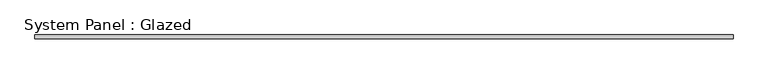
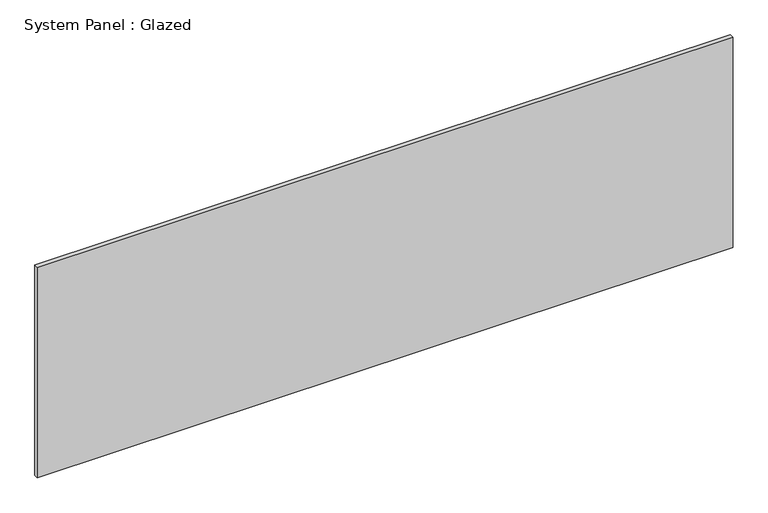
"""IFC4 building model written with IfcOpenShell, lengths in millimetres: plate geometry, System Panel : Glazed."""

from ifc_helpers import new_model, si_unit, origin, origin_with_axes, place, context, project, spatial, polyline, outline, extrude, source, transform, mapped, element, save


def system_panel_glazed_c13b8b16(model_context):
    return source(origin(), model_context, "Body", "SweptSolid", [
        extrude(outline(polyline([(2283.593154, 19.05), (-2283.593154, 19.05), (-2283.593154, 44.45), (2283.593154, 44.45), (2283.593154, 19.05)])), origin_with_axes(), (0.0, 0.0, 1.0), 1460.5),
    ])


if __name__ == "__main__":
    model = new_model("IFC4")
    model_context = context("Model", 3, world=origin())
    ifc_project = project(units=[si_unit("LENGTHUNIT", "METRE", prefix="MILLI")], contexts=[model_context])
    site = spatial("IfcSite", under=ifc_project)
    building = spatial("IfcBuilding", under=site)
    placement = place(None, origin())
    system_panel_glazed_shape = system_panel_glazed_c13b8b16(model_context)
    element("IfcPlate", 1, ObjectType="System Panel : Glazed", at=placement, inside=building, context=model_context, shape_type="MappedRepresentation", body=[
        mapped(system_panel_glazed_shape, transform((0.0, 0.0, 0.0), x_axis=(1.0, 0.0, 0.0), y_axis=(0.0, 1.0, 0.0), z_axis=(0.0, 0.0, 1.0))),
    ])
    save(model, "model.ifc")

# Revit data of these elements
# Type "System Panel : Glazed"
#   Construction Type Id = "GSP4R"
#   Analytic Construction = "1/8 in Pilkington single glazing"
#   Visual Light Transmittance = 0.9
#   Solar Heat Gain Coefficient = 0.86
#   Heat Transfer Coefficient (U) = 1.18115 BTU/(h·ft²·°F)
# Element 1 (IfcPlate, "System Panel : Glazed")
#   Materials on its faces: "Glass"
# Materials
#   "Glass": class "Glass", colour RGB 0 128 192, transparency 0.75, Description = "Soda Lime Glass", Cost = 0
